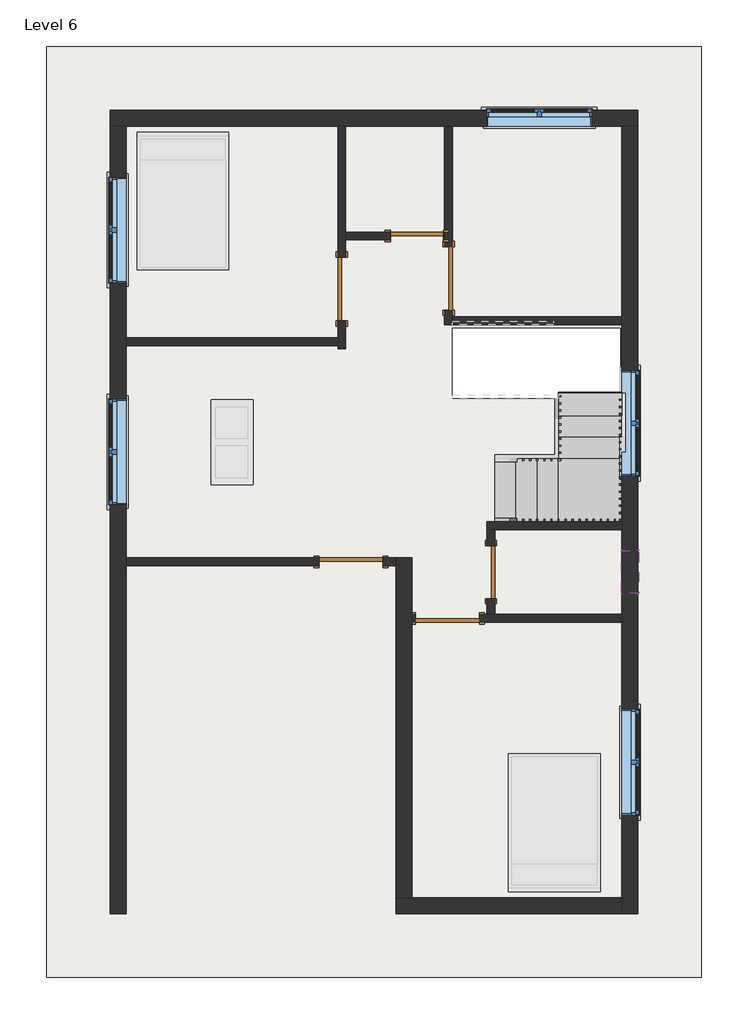
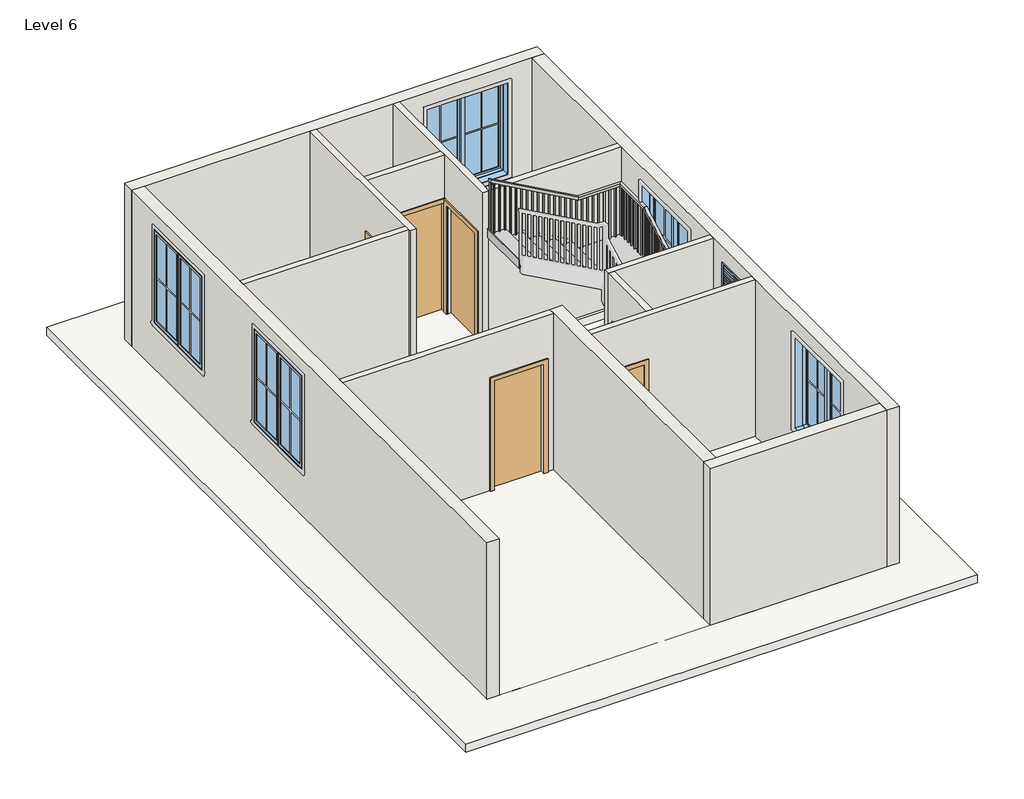
# One storey, part 1 of 2: 14 walls, 6 doors, 6 windows, 1 railing, 1 roof, 1 slab, 1 stair flight.
# Revit data of these elements (continued)
# Element 27 (IfcWindow, "Window-Casement-Double : WIN 5'")
#   Mark = "27"
#   Window Inset = 0' - 0"
#   Interior Wall Closure = 0' - 2 1/4"
#   Frame Extension = 0' - 0 1/4"
#   Exterior Wall Closure = 0' - 1 1/4"
#   Interior Trim Visibility = yes
#   Exterior Trim Visibility = yes
#   Phase Created = New Construction
#   Materials on its faces: "Wood - Stained", "Glass", "Clad - White"
# Element 28 (IfcWindow, "Window-Casement-Double : WIN 5'")
#   Mark = "28"
#   Window Inset = 0' - 0"
#   Interior Wall Closure = 0' - 2 1/4"
#   Frame Extension = 0' - 0 1/4"
#   Exterior Wall Closure = 0' - 1 1/4"
#   Interior Trim Visibility = yes
#   Exterior Trim Visibility = yes
#   Phase Created = New Construction
#   Materials on its faces: "Wood - Stained", "Glass", "Clad - White"
# Element 29 (IfcWindow, "Window-Casement-Double : WIN 5'")
#   Mark = "29"
#   Window Inset = 0' - 0"
#   Interior Wall Closure = 0' - 2 1/4"
#   Frame Extension = 0' - 0 1/4"
#   Exterior Wall Closure = 0' - 1 1/4"
#   Interior Trim Visibility = yes
#   Exterior Trim Visibility = yes
#   Phase Created = New Construction
#   Materials on its faces: "Wood - Stained", "Glass", "Clad - White"
# Element 30 (IfcWindow, "Window-Louvers : 24\" x 24\"")
#   Mark = "30"
#   Blade Width = 1' - 10 1/2"
#   Phase Created = New Construction
#   Materials on its faces: "Birch"
# Materials
#   "Door - Panel": class "Wood", colour RGB 210 159 95, transparency 0, Cost = 0
#   "Door - Frame": colour RGB 118 70 51, transparency 0, Cost = 0
#   "Wood - Stained": class "Wood", colour RGB 224 178 126, transparency 0, Cost = 0
#   "Glass": class "Glass", colour RGB 0 128 192, transparency 0.75, Description = "Soda Lime Glass", Cost = 0
#   "Clad - White": class "Wood", colour RGB 242 242 238, transparency 0, Cost = 0
#   "Birch": class "Wood", colour RGB 224 178 126, transparency 0, Description = "Betula Alleghaniensis", Cost = 0
#   "Default Roof": colour RGB 88 101 114, transparency 0, Cost = 0
#   "Default Floor": colour RGB 128 128 128, transparency 0, Cost = 0
#   "Default Wall": colour RGB 128 128 128, transparency 0, Cost = 0
#   "Copper": class "Metal", colour RGB 0 0 0, transparency 0, Description = "Copper, matte finish", Cost = 0
